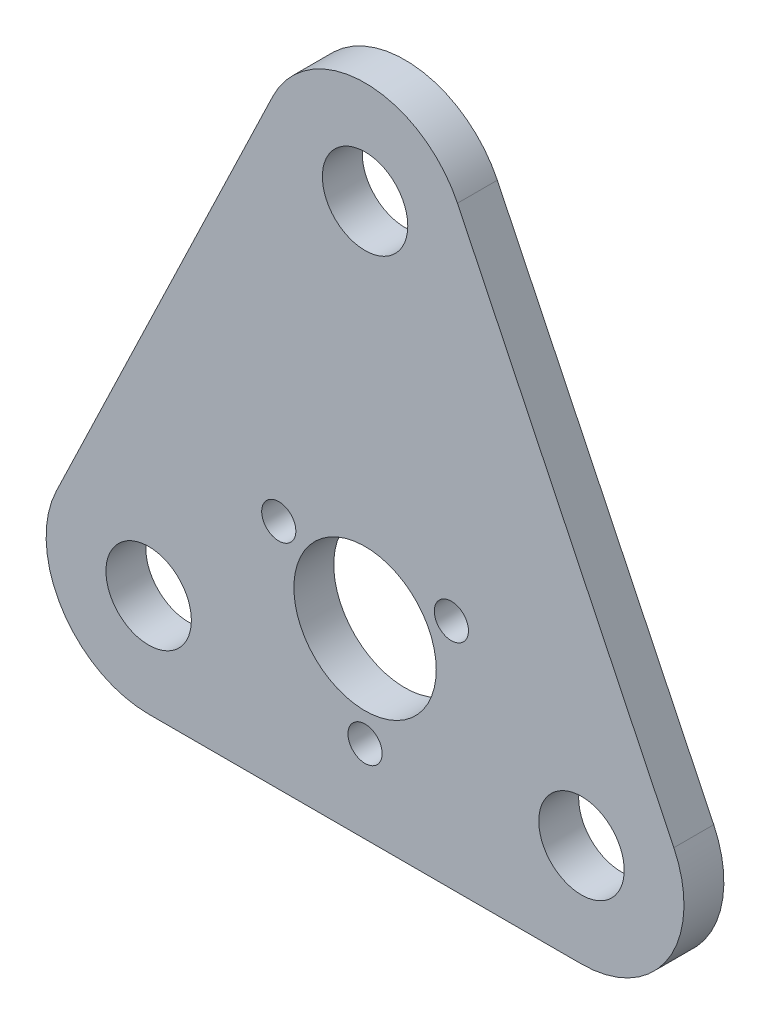
from build123d import *

# Parameters (mm, degrees)
PLATE_PROFILE_R         = 12.5
PLATE_PROFILE_R_2       = 3
PLATE_PROFILE_R_3       = 7.5
SUPPORT_PLATE_7MM_DEPTH = 7


with BuildPart() as part:
    # Plate Profile → Support Plate 7mm (new body)
    with BuildSketch(Plane.XY):
        with BuildLine():
            Line((-38, -32), (38, -32))
            ThreePointArc((38, -32), (53.238850443, -23.580054133), (54.221001351, -6.197493021))
            Line((54.221001351, -6.197493021), (16.221001351, 72.802506979))
            ThreePointArc((16.221001351, 72.802506979), (0, 83), (-16.221001351, 72.802506979))
            Line((-16.221001351, 72.802506979), (-54.221001351, -6.197493021))
            ThreePointArc((-54.221001351, -6.197493021), (-53.238850443, -23.580054133), (-38, -32))
        make_face()
        Circle(PLATE_PROFILE_R, mode=Mode.SUBTRACT)
        with Locations((0, -17.5)):
            Circle(PLATE_PROFILE_R_2, mode=Mode.SUBTRACT)
        with Locations((-15.155444566, 8.75)):
            Circle(PLATE_PROFILE_R_2, mode=Mode.SUBTRACT)
        with Locations((15.155444566, 8.75)):
            Circle(PLATE_PROFILE_R_2, mode=Mode.SUBTRACT)
        with Locations((-38, -14)):
            Circle(PLATE_PROFILE_R_3, mode=Mode.SUBTRACT)
        with Locations(Location((38, -14, 0), (0, 0, 180))):
            Circle(PLATE_PROFILE_R_3, mode=Mode.SUBTRACT)
        with Locations((0, 65)):
            Circle(PLATE_PROFILE_R_3, mode=Mode.SUBTRACT)
    extrude(amount=SUPPORT_PLATE_7MM_DEPTH)


solid = part.part
